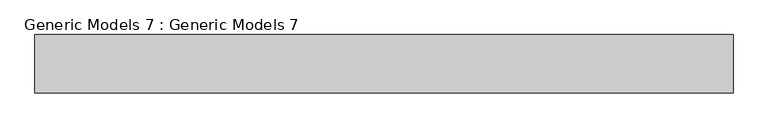
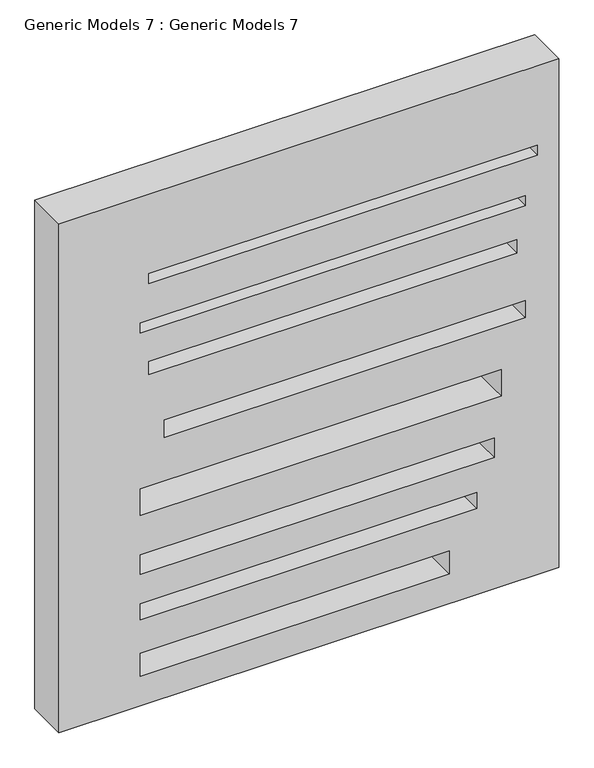
"""IFC4 building model written with IfcOpenShell, lengths in millimetres: proxy geometry, Generic Models 7 : Generic Models 7."""

from ifc_helpers import new_model, si_unit, frame, origin, place, context, project, spatial, polyline, outline, extrude, source, transform, mapped, element, save


def generic_models_7_generic_models_7_d72a22cb(model_context):
    return source(origin(), model_context, "Body", "SweptSolid", [
        extrude(outline(polyline([(-124.2050178, -11946.7297481), (3813.1326905, -11946.7297481), (3813.1326905, -15604.3297481), (-124.2050178, -15604.3297481), (-124.2050178, -11946.7297481)]), holes=[polyline([(3121.7358297, -12102.0772922), (3121.7358297, -14945.6063069), (3200.4, -14945.6063069), (3200.4, -12102.0772922), (3121.7358297, -12102.0772922)]), polyline([(2761.5855319, -12189.8356484), (2761.5855319, -15009.2356484), (2837.7855319, -15009.2356484), (2837.7855319, -12189.8356484), (2761.5855319, -12189.8356484)]), polyline([(2417.5572071, -12253.2063069), (2417.5572071, -14945.6063069), (2519.1572071, -14945.6063069), (2519.1572071, -12253.2063069), (2417.5572071, -12253.2063069)]), polyline([(1892.6029001, -12189.8356484), (1892.6029001, -14833.9753019), (2026.956054, -14833.9753019), (2026.956054, -12189.8356484), (1892.6029001, -12189.8356484)]), polyline([(1349.7788075, -12367.6356484), (1349.7788075, -15009.2356484), (1552.9788075, -15009.2356484), (1552.9788075, -12367.6356484), (1349.7788075, -12367.6356484)]), polyline([(891.3275883, -12418.4356484), (891.3275883, -15009.2356484), (1043.7275883, -15009.2356484), (1043.7275883, -12418.4356484), (891.3275883, -12418.4356484)]), polyline([(539.1898462, -12545.4356484), (539.1898462, -15009.2356484), (666.1898462, -15009.2356484), (666.1898462, -12545.4356484), (539.1898462, -12545.4356484)]), polyline([(103.5555261, -12748.6356484), (103.5555261, -15009.2356484), (281.3555261, -15009.2356484), (281.3555261, -12748.6356484), (103.5555261, -12748.6356484)])]), frame((0.0, -4864.6088252, 0.0), z_axis=(0.0, 1.0, 0.0), x_axis=(0.0, 0.0, 1.0)), (0.0, 0.0, 1.0), 304.8),
    ])


if __name__ == "__main__":
    model = new_model("IFC4")
    model_context = context("Model", 3, world=origin())
    ifc_project = project(units=[si_unit("LENGTHUNIT", "METRE", prefix="MILLI")], contexts=[model_context])
    site = spatial("IfcSite", under=ifc_project)
    building = spatial("IfcBuilding", under=site)
    placement = place(None, origin())
    generic_models_7_generic_models_7_shape = generic_models_7_generic_models_7_d72a22cb(model_context)
    element("IfcBuildingElementProxy", 1, Name="Generic Models 7 : Generic Models 7", ObjectType="Generic Models 7 : Generic Models 7", at=placement, inside=building, context=model_context, shape_type="MappedRepresentation", body=[
        mapped(generic_models_7_generic_models_7_shape, transform((0.0, 0.0, 0.0), x_axis=(1.0, 0.0, 0.0), y_axis=(0.0, 1.0, 0.0), z_axis=(0.0, 0.0, 1.0))),
    ])
    save(model, "model.ifc")
